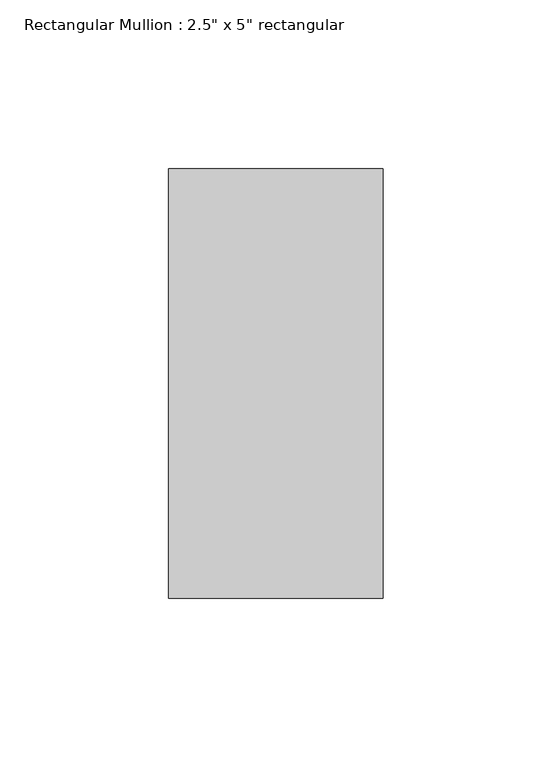
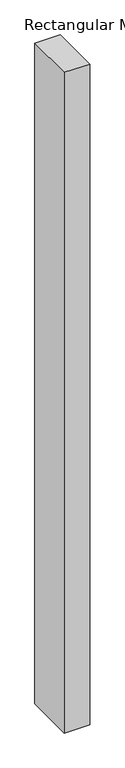
"""IFC4 building model written with IfcOpenShell, lengths in millimetres: member geometry."""

from ifc_helpers import new_model, si_unit, frame, origin, place, context, project, spatial, polyline, outline, extrude, source, transform, mapped, element, save


def member_bc773a83(model_context):
    return source(origin(), model_context, "Body", "SweptSolid", [
        extrude(outline(polyline([(31.75, 63.5), (31.75, -63.5), (-31.75, -63.5), (-31.75, 63.5), (31.75, 63.5)])), frame((0.0, 0.0, -1747.5125275), z_axis=(0.0, 0.0, 1.0), x_axis=(1.0, 0.0, 0.0)), (0.0, 0.0, 1.0), 1747.5125275),
    ])


if __name__ == "__main__":
    model = new_model("IFC4")
    model_context = context("Model", 3, world=origin())
    ifc_project = project(units=[si_unit("LENGTHUNIT", "METRE", prefix="MILLI")], contexts=[model_context])
    site = spatial("IfcSite", under=ifc_project)
    building = spatial("IfcBuilding", under=site)
    placement = place(None, origin())
    member_shape = member_bc773a83(model_context)
    element("IfcMember", 1, ObjectType="Rectangular Mullion : 2.5\" x 5\" rectangular", at=placement, inside=building, context=model_context, shape_type="MappedRepresentation", body=[
        mapped(member_shape, transform((0.0, 0.0, 0.0), x_axis=(1.0, 0.0, 0.0), y_axis=(0.0, 1.0, 0.0), z_axis=(0.0, 0.0, 1.0))),
    ])
    save(model, "model.ifc")

# Revit data of these elements
# Type "Rectangular Mullion : 2.5\" x 5\" rectangular"
#   built-in parameter 1007304 = 0.416667 (stored number, unit not read)
#   built-in parameter 1007301 = 0.104167 (stored number, unit not read)
#   built-in parameter 1007300 = 0.104167 (stored number, unit not read)
# Element 1 (IfcMember, "Rectangular Mullion : 2.5\" x 5\" rectangular")
#   Materials on its faces: "Aluminum"
# Materials
#   "Aluminum": class "Metal", colour RGB 247 247 247, transparency 0, Description = "Aluminum 6061", Cost = 0
